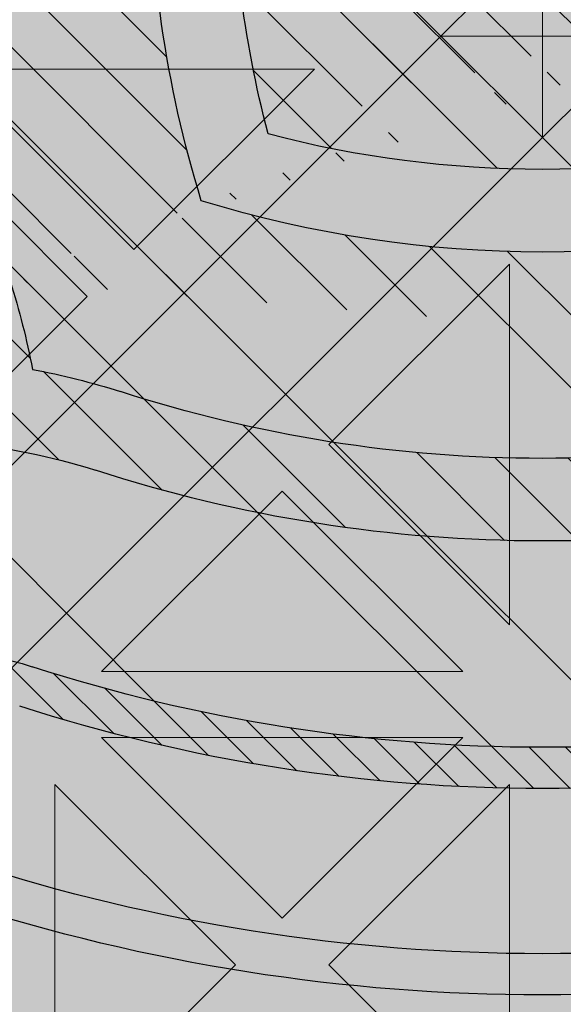
# Model space of a CAD drawing. Units: inches. Extents: x 844 to 2234, y 346 to 1084.
# Tile 28 of 93: x 1255.358 to 1257.455, y 687.38 to 691.183. Entities that reach past the tile are written whole.
import ezdxf

# ---------------------------------------------------------------- set-up
doc = ezdxf.new("R2010")
doc.units = ezdxf.units.IN
doc.header["$MEASUREMENT"] = 0
doc.layers.add('furniture', color=8, linetype='Continuous', lineweight=18)
doc.layers.add('RA-AP-01$0$INT', color=35, linetype='Continuous', lineweight=5)
doc.layers.add('RA-AP-01$0$FURN', color=3, linetype='Continuous')
doc.layers.add('RA-AP-01$0$WOOD', color=64, linetype='Continuous')

# ---------------------------------------------------------------- blocks, each defined once
blk = doc.blocks.new('A$C18D01794')
at = {"layer": 'RA-AP-01$0$INT'}
h = blk.add_hatch(color=256, dxfattribs=at)
h.paths.add_polyline_path([(4.585917135068449, -6.356712009588271), (4.555206456959269, -6.35671200958746), (4.555206456959137, -6.387422687716308), (4.874495778835233, -6.706712009592356), (4.90520645695423, -6.676001331474049)])
h.paths.add_polyline_path([(5.255206456948813, -6.387422687716306), (5.255206456948682, -6.356712009605972), (5.224495778822613, -6.356712009605161), (4.905206456953498, -6.676001331474273), (4.935917135072151, -6.706712009592924)])
h.paths.add_polyline_path([(4.935917135072559, -6.706712009592068), (4.905206456953564, -6.737422687710376), (5.255206456951813, -7.087422687708613), (5.255206456951549, -7.026001331471008)])
h.paths.add_polyline_path([(4.555206456956399, -7.026001331471013), (4.555206456956134, -7.087422687708616), (4.905206456953821, -6.737422687710943), (4.874495778835166, -6.70671200959229)])
h = blk.add_hatch(color=256, dxfattribs=at)
h.paths.add_polyline_path([(4.585917135068448, -6.356712009588273), (4.614201406330596, -6.356712009589021), (4.668846067270487, -6.411356670531338), (4.723490728212344, -6.356712009591912), (4.771774999457151, -6.35671200959319), (4.826419660396886, -6.411356670535356), (4.862780050090322, -6.374996280843536), (4.844495778842715, -6.356712009595112), (4.862780050090411, -6.356712009595595), (4.905206456960182, -6.399138416468211), (4.947632863832445, -6.356712009597838), (4.965917135079675, -6.356712009598322), (4.947632863831759, -6.374996280845421), (4.983993253523576, -6.411356670538857), (5.038637914464627, -6.356712009600247), (5.08692218571208, -6.356712009601523), (5.141566846649976, -6.411356670541852), (5.196211507589851, -6.356712009604411), (5.224495778822615, -6.356712009605161), (4.905206456953975, -6.676001331473793)])
h.paths.add_polyline_path([(4.895206456956031, -6.637717060225675), (4.895206456958921, -6.528427738347902), (4.840561796018589, -6.583072399285802)], flags=16)
h.paths.add_polyline_path([(4.915206456955638, -6.637717060226121), (4.969851117895509, -6.583072399288678), (4.915206456957609, -6.528427738348344)], flags=16)
h.paths.add_polyline_path([(4.826419660395175, -6.568930263661755), (4.881064321335613, -6.514285602723745), (4.771774999456703, -6.514285602720857)], flags=16)
h.paths.add_polyline_path([(4.983993253519558, -6.568930263665262), (5.038637914460456, -6.514285602726792), (4.929348592581548, -6.514285602724816)], flags=16)
h.paths.add_polyline_path([(4.881064321336025, -6.494285602723742), (4.826419660397532, -6.439640941782821), (4.771774999457062, -6.494285602720859)], flags=16)
h.paths.add_polyline_path([(4.929348592582019, -6.494285602724817), (5.038637914460982, -6.494285602726792), (4.983993253522945, -6.439640941786327)], flags=16)
h.paths.add_polyline_path([(4.895206456960191, -6.480143467100443), (4.895206456962115, -6.407422687715913), (4.876922185715016, -6.389138416467584), (4.840561796021581, -6.425498806159401)], flags=16)
h.paths.add_polyline_path([(4.915206456958487, -6.480143467100889), (4.969851117899527, -6.425498806162279), (4.933490728206909, -6.389138416468043), (4.9152064569598, -6.40742268771434)], flags=16)
h.paths.add_polyline_path([(4.757632863832376, -6.480143467096812), (4.812277524772842, -6.425498806158772), (4.757632863834348, -6.370854145217844)], flags=16)
h.paths.add_polyline_path([(4.737632863832376, -6.480143467096286), (4.737632863834348, -6.370854145217375), (4.682988202893906, -6.425498806155385)], flags=16)
h.paths.add_polyline_path([(5.05278005008503, -6.480143467103376), (5.052780050087917, -6.370854145224413), (4.998135389146995, -6.425498806162908)], flags=16)
h.paths.add_polyline_path([(5.072780050085024, -6.480143467103744), (5.127424711025931, -6.42549880616527), (5.072780050087916, -6.370854145224832)], flags=16)
h.paths.add_polyline_path([(4.935917135072783, -6.706712009592292), (5.255206456948811, -6.387422687716309), (5.255206456948932, -6.415706958964177), (5.200561796010279, -6.470351619902839), (5.255206456949403, -6.524996280841948), (5.25520645694961, -6.5732805520894), (5.200561796009787, -6.627925213029239), (5.236922185702417, -6.664285602721864), (5.255206456949919, -6.646001331474357), (5.255206456949998, -6.664285602721898), (5.212780050078687, -6.706712009592262), (5.25520645695036, -6.749138416463932), (5.255206456950438, -6.767422687711313), (5.236922185702424, -6.749138416463297), (5.200561796009796, -6.785498806155928), (5.255206456950753, -6.840143467096874), (5.25520645695096, -6.888427738341682), (5.200561796010322, -6.943072399282328), (5.255206456951428, -6.997717060223427), (5.255206456951547, -7.026001331471006)])
h.paths.add_polyline_path([(5.042988202883395, -6.785498806155427), (5.097632863823085, -6.840143467095101), (5.097632863822622, -6.730854145216193)], flags=16)
h.paths.add_polyline_path([(5.028846067259663, -6.771356670531693), (5.083490728198774, -6.716712009592573), (4.974201406321001, -6.716712009593042)], flags=16)
h.paths.add_polyline_path([(5.117632863823087, -6.840143467095186), (5.172277524762331, -6.785498806155926), (5.11763286382262, -6.730854145216225)], flags=16)
h.paths.add_polyline_path([(5.08349072819877, -6.696712009593886), (5.028846067259652, -6.642067348654775), (4.974201406320998, -6.696712009593438)], flags=16)
h.paths.add_polyline_path([(5.131774999446817, -6.854285602718917), (5.186419660386065, -6.799640941779662), (5.241064321325782, -6.854285602719365)], flags=17)
h.paths.add_polyline_path([(5.131774999446228, -6.716712009592374), (5.186419660386065, -6.771356670532194), (5.222780050079488, -6.734996280838764), (5.204495778832781, -6.716712009592063)], flags=16)
h.paths.add_polyline_path([(5.097632863822613, -6.682569873970264), (5.097632863823061, -6.573280552091354), (5.042988202883383, -6.627925213031044)], flags=16)
h.paths.add_polyline_path([(5.131774999446899, -6.874285602718915), (5.241064321325809, -6.874285602719364), (5.186419660386591, -6.928930263658598)], flags=17)
h.paths.add_polyline_path([(5.131774999446226, -6.696712009594078), (5.204495778830767, -6.696712009594374), (5.22278005007868, -6.67842773834687), (5.186419660386049, -6.642067348654249)], flags=16)
h.paths.add_polyline_path([(5.11763286382262, -6.682569873970225), (5.17227752476232, -6.627925213030515), (5.117632863823064, -6.573280552091267)], flags=16)
h.paths.add_polyline_path([(5.186419660386069, -6.613783077405491), (5.241064321325754, -6.559138416465795), (5.131774999446791, -6.559138416466263)], flags=16)
h.paths.add_polyline_path([(5.131774999446872, -6.539138416466263), (5.24106432132578, -6.539138416465794), (5.186419660386554, -6.484493755526573)], flags=16)
h.paths.add_polyline_path([(5.255206456951811, -7.08742268770861), (5.255206456951895, -7.106712009588038), (4.555206456956052, -7.106712009588038), (4.555206456956136, -7.087422687708617), (4.905206456953973, -6.737422687710788)])
h.paths.add_polyline_path([(4.983993253513404, -6.8444937555241), (4.92934859257295, -6.899138416462108), (5.03863791445186, -6.899138416465014)], flags=16)
h.paths.add_polyline_path([(4.969851117889988, -6.83035161990006), (4.915206456952556, -6.775706958960171), (4.915206456949648, -6.884996280837944)], flags=16)
h.paths.add_polyline_path([(4.929348592572535, -6.919138416462105), (4.983993253511019, -6.973783077403037), (5.038637914451496, -6.919138416465012)], flags=16)
h.paths.add_polyline_path([(5.052780050074912, -6.93328055208906), (4.998135389134438, -6.987925213027088), (5.052780050072919, -7.042569873968025)], flags=16)
h.paths.add_polyline_path([(5.07278005007491, -6.933280552089588), (5.072780050072918, -7.042569873968497), (5.127424711013374, -6.987925213030498)], flags=16)
h.paths.add_polyline_path([(4.89520645695295, -6.775706958959721), (4.840561796013067, -6.830351619897157), (4.895206456950961, -6.884996280837494)], flags=16)
h.paths.add_polyline_path([(4.915206456948365, -6.933280552085403), (4.915206456946434, -7.006001331471951), (4.933490728192729, -7.024285602719066), (4.969851117886972, -6.987925213026453)], flags=16)
h.paths.add_polyline_path([(4.881064321327021, -6.899138416461022), (4.82641966038902, -6.84449375552057), (4.771774999448108, -6.899138416459029)], flags=16)
h.paths.add_polyline_path([(4.895206456950073, -6.933280552084951), (4.840561796009022, -6.987925213023558), (4.876922185700835, -7.024285602716997), (4.895206456948749, -7.006001331469487)], flags=16)
h.paths.add_polyline_path([(4.983993253510392, -7.0020673486505), (4.947632863816944, -7.038427738342319), (4.965917135064043, -7.05671200959023), (5.038637914448995, -7.056712009591555)], flags=16)
h.paths.add_polyline_path([(4.881064321326543, -6.91913841646102), (4.771774999447578, -6.919138416459031), (4.826419660385607, -6.973783077399508)], flags=16)
h.paths.add_polyline_path([(4.905206456946447, -7.014285602717636), (4.862780050074785, -7.056712009588352), (4.947632863816685, -7.056712009589775)], flags=16)
h.paths.add_polyline_path([(5.14156684663679, -7.002067348654549), (5.086922185696452, -7.056712009592438), (5.196211507574223, -7.056712009594425)], flags=16)
h.paths.add_polyline_path([(4.8264196603837, -7.002067348646972), (4.771774999442643, -7.056712009585575), (4.8444957788276, -7.056712009587508), (4.862780050075511, -7.038427738340416)], flags=16)
h.paths.add_polyline_path([(4.812277524760289, -6.98792521302292), (4.757632863822258, -6.933280552082447), (4.757632863819352, -7.042569873961408)], flags=16)
h.paths.add_polyline_path([(4.73763286382226, -6.933280552082079), (4.682988202881349, -6.987925213020536), (4.737632863819352, -7.04256987396099)], flags=16)
h.paths.add_polyline_path([(4.723490728195188, -7.056712009584289), (4.668846067257299, -7.002067348643949), (4.614201406317417, -7.056712009581383)], flags=16)
h.paths.add_polyline_path([(4.597632863829262, -6.706712009592262), (4.555206456957951, -6.664285602721896), (4.555206456958029, -6.646001331474357), (4.573490728205535, -6.664285602721864), (4.609851117898167, -6.627925213029238), (4.555206456958338, -6.573280552089402), (4.555206456958546, -6.524996280841952), (4.60985111789767, -6.470351619902839), (4.555206456959015, -6.415706958964177), (4.555206456959138, -6.387422687716309), (4.874495778835167, -6.70671200959229), (4.5552064569564, -7.026001331471015), (4.555206456956523, -6.997717060223433), (4.609851117897629, -6.94307239928233), (4.555206456956988, -6.888427738341681), (4.555206456957198, -6.840143467096881), (4.609851117898153, -6.78549880615593), (4.573490728205528, -6.749138416463297), (4.555206456957507, -6.76742268771132), (4.555206456957585, -6.749138416463933)])
h.paths.add_polyline_path([(4.712780050085332, -6.730854145216195), (4.712780050084863, -6.840143467095105), (4.767424711024555, -6.785498806155427)], flags=16)
h.paths.add_polyline_path([(4.726922185709173, -6.716712009592573), (4.781566846648288, -6.771356670531693), (4.836211507586949, -6.716712009593043)], flags=16)
h.paths.add_polyline_path([(4.692780050085327, -6.730854145216225), (4.638135389145619, -6.785498806155928), (4.692780050084865, -6.840143467095185)], flags=16)
h.paths.add_polyline_path([(4.726922185709182, -6.696712009593886), (4.836211507586949, -6.696712009593436), (4.7815668466483, -6.642067348654773)], flags=16)
h.paths.add_polyline_path([(4.678637914461726, -6.71671200959237), (4.605917135075169, -6.716712009592063), (4.587632863828464, -6.734996280838766), (4.623993253521887, -6.771356670532195)], flags=16)
h.paths.add_polyline_path([(4.712780050085336, -6.68256987397026), (4.767424711024568, -6.627925213031042), (4.71278005008489, -6.573280552091352)], flags=16)
h.paths.add_polyline_path([(4.678637914461726, -6.696712009594076), (4.623993253521899, -6.642067348654247), (4.587632863829271, -6.67842773834687), (4.605917135077185, -6.696712009594376)], flags=16)
h.paths.add_polyline_path([(4.692780050085336, -6.682569873970228), (4.692780050084889, -6.573280552091267), (4.638135389145632, -6.627925213030515)], flags=16)
h.paths.add_polyline_path([(4.623993253521885, -6.799640941779662), (4.678637914461131, -6.854285602718915), (4.56934859258217, -6.854285602719365)], flags=17)
h.paths.add_polyline_path([(4.623993253521901, -6.613783077405509), (4.678637914461158, -6.559138416466263), (4.569348592582195, -6.559138416465795)], flags=16)
h.paths.add_polyline_path([(4.678637914461051, -6.874285602718915), (4.623993253521361, -6.928930263658598), (4.569348592582143, -6.874285602719364)], flags=17)
h.paths.add_polyline_path([(4.678637914461076, -6.539138416466263), (4.623993253521399, -6.484493755526573), (4.569348592582167, -6.539138416465796)], flags=16)
h = blk.add_hatch(color=256, dxfattribs=at)
h.paths.add_polyline_path([(4.969851117891331, -6.583072399286455), (4.915206456952669, -6.63771706022511), (4.915206456952222, -6.528427738347337)])
h.paths.add_polyline_path([(4.895206456953064, -6.637717060225108), (4.840561796014413, -6.583072399286448), (4.895206456953533, -6.528427738347335)])
h.paths.add_polyline_path([(4.826419660390684, -6.568930263662714), (4.771774999451003, -6.514285602723024), (4.881064321329913, -6.514285602723489)])
h.paths.add_polyline_path([(4.881064321329884, -6.494285602723492), (4.771774999450921, -6.494285602723024), (4.82641966039018, -6.439640941783778)])
h.paths.add_polyline_path([(4.895206456953734, -6.48014346709988), (4.840561796013912, -6.425498806160046), (4.876922185707337, -6.389138416466622), (4.895206456954043, -6.40742268771333)])
h.paths.add_polyline_path([(4.862780050082808, -6.374996280843689), (4.826419660390178, -6.411356670536314), (4.771774999450351, -6.356712009596481), (4.844495778835303, -6.356712009596181)])
h.paths.add_polyline_path([(4.812277524766446, -6.425498806160041), (4.757632863827191, -6.480143467099289), (4.757632863826741, -6.370854145220329)])
h.paths.add_polyline_path([(4.737632863827191, -6.480143467099214), (4.682988202887508, -6.425498806159518), (4.737632863826743, -6.370854145220299)])
h.paths.add_polyline_path([(4.668846067263777, -6.41135667053579), (4.614201406325123, -6.356712009597128), (4.723490728202894, -6.356712009596675)])
h.paths.add_polyline_path([(4.905206456953846, -6.399138416467422), (4.862780050082654, -6.356712009596229), (4.947632863824561, -6.356712009595756)])
h.paths.add_polyline_path([(4.915206456952028, -6.480143467099882), (4.91520645695173, -6.407422687715346), (4.933490728199234, -6.389138416467428), (4.96985111789186, -6.425498806160055)])
h.paths.add_polyline_path([(5.038637914454841, -6.494285602723048), (4.929348592575874, -6.494285602723497), (4.983993253515593, -6.439640941783787)])
h.paths.add_polyline_path([(4.983993253515065, -6.568930263662725), (4.929348592575849, -6.514285602723495), (5.038637914454755, -6.514285602723045)])
h.paths.add_polyline_path([(5.052780050079843, -6.480143467099317), (4.998135389140595, -6.425498806160058), (5.052780050080309, -6.370854145220356)])
h.paths.add_polyline_path([(4.983993253516868, -6.411356670536324), (4.947632863824241, -6.374996280843694), (4.965917135071747, -6.356712009596188), (5.038637914456701, -6.356712009596504)])
h.paths.add_polyline_path([(5.127424711019533, -6.425498806159557), (5.072780050079843, -6.480143467099239), (5.07278005008031, -6.370854145220326)])
h.paths.add_polyline_path([(5.141566846643269, -6.411356670535829), (5.086922185704154, -6.356712009596707), (5.196211507581929, -6.356712009597176)])
h = blk.add_hatch(color=256, dxfattribs=at)
h.paths.add_polyline_path([(5.028846067259997, -6.642067348655121), (4.974201406321342, -6.696712009593783), (5.083490728199115, -6.69671200959423)])
h.paths.add_polyline_path([(4.974201406321344, -6.716712009593388), (5.028846067260004, -6.771356670532039), (5.083490728199117, -6.716712009592919)])
h.paths.add_polyline_path([(5.042988202883738, -6.785498806155768), (5.097632863823428, -6.840143467095449), (5.097632863822963, -6.73085414521654)])
h.paths.add_polyline_path([(5.117632863822961, -6.730854145216568), (5.117632863823428, -6.840143467095531), (5.172277524762674, -6.785498806156272)])
h.paths.add_polyline_path([(5.131774999446572, -6.716712009592718), (5.186419660386406, -6.77135667053254), (5.222780050079831, -6.734996280839116), (5.204495778833122, -6.716712009592409)])
h.paths.add_polyline_path([(5.236922185702764, -6.749138416463644), (5.200561796010139, -6.785498806156274), (5.255206456949971, -6.840143467096101), (5.255206456950271, -6.76742268771115)])
h.paths.add_polyline_path([(5.186419660386412, -6.799640941780006), (5.131774999447164, -6.854285602719262), (5.241064321326123, -6.854285602719711)])
h.paths.add_polyline_path([(5.131774999447238, -6.874285602719261), (5.186419660386934, -6.928930263658944), (5.241064321326153, -6.874285602719709)])
h.paths.add_polyline_path([(5.200561796010663, -6.943072399282675), (5.255206456949324, -6.997717060221329), (5.255206456949777, -6.888427738343558)])
h.paths.add_polyline_path([(5.21278005007903, -6.706712009592607), (5.255206456950223, -6.749138416463798), (5.255206456950696, -6.664285602721891)])
h.paths.add_polyline_path([(5.13177499944657, -6.696712009594424), (5.204495778831106, -6.696712009594723), (5.222780050079024, -6.678427738347219), (5.186419660386397, -6.642067348654592)])
h.paths.add_polyline_path([(5.117632863823405, -6.573280552091611), (5.117632863822955, -6.682569873970578), (5.172277524762665, -6.627925213030859)])
h.paths.add_polyline_path([(5.042988202883727, -6.627925213031387), (5.097632863822957, -6.682569873970603), (5.097632863823407, -6.573280552091697)])
h.paths.add_polyline_path([(5.131774999447135, -6.559138416466609), (5.186419660386394, -6.613783077405857), (5.241064321326097, -6.559138416466144)])
h.paths.add_polyline_path([(5.200561796010128, -6.627925213029584), (5.236922185702758, -6.664285602722211), (5.255206456950264, -6.646001331474705), (5.255206456949948, -6.573280552089752)])
h.paths.add_polyline_path([(5.186419660386895, -6.484493755526919), (5.131774999447213, -6.539138416466609), (5.241064321326127, -6.539138416466142)])
h.paths.add_polyline_path([(5.200561796010624, -6.470351619903183), (5.255206456949745, -6.524996280842298), (5.255206456949276, -6.415706958964523)])
h = blk.add_hatch(color=256, dxfattribs=at)
h.paths.add_polyline_path([(4.905206456953579, -6.70671200959253), (4.905206456953751, -6.676001331474523), (4.874495778835229, -6.706712009592358)])
h.paths.add_polyline_path([(4.935917135071924, -6.706712009592703), (4.905206456953583, -6.706712009592529), (4.90520645695341, -6.737422687710532)])
h = blk.add_hatch(color=256, dxfattribs=at)
h.paths.add_polyline_path([(4.905206456953409, -6.737422687710532), (4.90520645695358, -6.706712009592529), (4.874495778835235, -6.706712009592359)])
h.paths.add_polyline_path([(4.935917135071928, -6.706712009592703), (4.905206456953754, -6.676001331474527), (4.905206456953582, -6.706712009592529)])
for p, q in [((4.905206456953975, -6.676001331473793), (4.585917135071132, -6.356712009590955)), ((4.905206456953975, -6.676001331473793), (5.224495778822613, -6.356712009605161)), ((5.052780050087917, -6.370854145224413), (4.998135389146995, -6.425498806162908)), ((5.052780050085028, -6.480143467103376), (5.052780050087917, -6.370854145224413)), ((4.969851117899529, -6.425498806162279), (4.93349072820771, -6.389138416468842)), ((4.935917135072783, -6.706712009592292), (5.255206456948813, -6.387422687716307)), ((4.9152064569598, -6.407422687715939), (4.915206456958485, -6.480143467100891)), ((4.915206456958485, -6.480143467100891), (4.969851117899529, -6.425498806162277)), ((5.052780050085028, -6.480143467103376), (4.998135389146995, -6.425498806162908)), ((4.92934859258202, -6.494285602724817), (4.983993253522945, -6.439640941786326)), ((5.038637914460983, -6.494285602726792), (4.983993253522945, -6.439640941786326)), ((5.038637914460983, -6.494285602726792), (4.92934859258202, -6.494285602724817)), ((4.929348592581546, -6.514285602724816), (4.983993253519556, -6.568930263665262)), ((5.038637914460456, -6.514285602726792), (4.929348592581546, -6.514285602724816)), ((4.983993253519558, -6.56893026366526), (5.038637914460456, -6.514285602726792)), ((4.915206456957613, -6.52842773834835), (4.969851117895507, -6.583072399288678)), ((4.915206456957609, -6.528427738348348), (4.915206456955636, -6.637717060226119)), ((5.042988202883385, -6.627925213031041), (5.097632863823062, -6.573280552091352)), ((4.915206456955636, -6.637717060226119), (4.969851117895507, -6.583072399288678)), ((5.097632863822615, -6.682569873970262), (5.042988202883383, -6.627925213031042)), ((4.974201406320999, -6.696712009593436), (5.028846067259652, -6.642067348654775)), ((5.083490728198769, -6.696712009593882), (5.028846067259652, -6.642067348654775)), ((4.874495778835233, -6.706712009592356), (4.905206456953753, -6.676001331474525)), ((4.935917135071927, -6.706712009592701), (4.905206456953751, -6.676001331474525)), ((4.905206456953753, -6.676001331474525), (4.905206456953409, -6.737422687710532)), ((5.08349072819877, -6.696712009593886), (4.974201406320999, -6.696712009593436)), ((4.874495778835233, -6.706712009592358), (4.935917135071925, -6.706712009592703)), ((4.935917135071927, -6.706712009592701), (4.905206456953407, -6.737422687710532)), ((4.935917135072783, -6.706712009592292), (5.255206456951548, -7.026001331471007))]:
    blk.add_line(p, q, dxfattribs=at)
blk = doc.blocks.new('A$C32926AE1')
at = {"layer": 'RA-AP-01$0$FURN'}
h = blk.add_hatch(dxfattribs=at)
h.set_pattern_fill('ANSI31', color=256, scale=0.1, style=0)
h.set_pattern_definition([(45, (0, 0), (-0.0088388347648318, 0.0088388347648318), [])])
edge = h.paths.add_edge_path(flags=16)
edge.add_arc((4.904771284329206, 4.246793130718756), 0.2603971832811541, 75.22398030683196, 104.7760196931204)
edge.add_arc((4.904771284329206, 4.246793130718756), 0.2603971832811541, 75.223980306832, 104.77601969312039, ccw=False)
edge = h.paths.add_edge_path(flags=16)
edge.add_arc((4.904771284329206, 4.067062675376612), 0.2603971832811541, 255.2239803068796, 284.776019693168)
edge.add_arc((4.904771284329206, 4.067062675376612), 0.2603971832811541, 255.22398030687958, 284.77601969316805, ccw=False)
edge = h.paths.add_edge_path(flags=0)
edge.add_arc((4.904771284329206, 4.067062675376612), 0.2603971832811541, 255.2239803068796, 284.776019693168)
edge.add_arc((4.904771284329206, 4.067062675376612), 0.2603971832811541, 255.22398030687958, 284.77601969316805, ccw=False)
edge = h.paths.add_edge_path(flags=0)
edge.add_arc((4.904771284329206, 4.067062675376612), 0.2603971832811541, 255.2239803068796, 284.776019693168)
edge.add_arc((4.904771284329206, 4.067062675376612), 0.2603971832811541, 255.22398030687958, 284.77601969316805, ccw=False)
edge = h.paths.add_edge_path()
edge.add_arc((4.604388392048174, 4.588829985554312), 0.1599999999999918, 342.3781640246255, 354.4317409793762)
edge.add_arc((5.090145208887507, 4.43216705527679), 0.3503971832811637, 162.0091218307731, 180.3186872093483)
edge.add_arc((5.205154176610243, 4.588829985554953), 0.1599999999999917, 185.5682590208461, 197.6218359767349)
edge.add_arc((4.904771284329229, 4.246793130718735), 0.3503971832811761, 72.00912183053516, 107.9908781690354)
edge.add_arc((9.535952835716557, 4.28682295566602), 4.798342501046485, 178.2875002453811, 181.5576802719453)
edge.add_arc((4.719397359771122, 4.43216705527679), 0.3503971832811637, 359.6813127906516, 377.9908781692269)
edge.add_arc((9.535967292294904, 4.286822350292874), 4.778371420254705, 178.2965938931842, 181.5667745797229)
edge.add_arc((4.719397359771122, 4.43216705527679), 0.3303971832811637, 359.6813127906516, 377.9908781692269)
edge.add_arc((0.2735752763637294, 4.286822350292874), 4.7783714202547, 358.4332254202771, 361.7034061068158)
edge.add_arc((5.061434214606998, 4.732549947558029), 0.1600000000000254, 252.3781640250584, 264.4317409792362)
edge.add_arc((4.748108354051257, 4.732549947558012), 0.1600000000000541, 275.5682590208426, 287.6218359759532)
edge.add_arc((4.604388392048115, 4.588829985554317), 0.1800000000000505, 342.3567572500182, 349.3735009646207)
edge.add_arc((5.205154176610254, 4.588829985554976), 0.1800000000000069, 190.6264990356027, 197.6432427513933)
edge.add_arc((5.061434214607106, 4.732549947558013), 0.1800000000000424, 252.3567572496606, 259.3735009644582)
edge.add_arc((4.904771284329208, 4.246793130718737), 0.3303971832811676, 71.99844483668534, 108.0015551637021)
edge.add_arc((4.748108354051414, 4.732549947558045), 0.1800000000000547, 280.6264990355479, 287.6432427495938)
edge.add_arc((5.090145208887514, 4.432167055276789), 0.2803971832811691, 162.8706300666893, 180.816523289902)
edge.add_arc((4.719397359771136, 4.432167055276689), 0.2803971832811534, 359.183476710103, 377.1293699333214)
edge.add_arc((4.904771284329222, 4.246793130718737), 0.2803971832811769, 72.87063006672916, 107.1293699332334)
edge.add_arc((5.090145208887522, 4.432167055276788), 0.2603971832811776, 165.2239803068007, 180.9953123810312)
edge.add_arc((4.719397359771141, 4.432167055276699), 0.2603971832811458, 359.0046876189768, 374.7760196932087)
edge.add_arc((5.090145208887507, 4.43216705527679), 0.3303971832811637, 162.0091218307731, 180.3186872093483)
edge.add_arc((9.53595427642584, 4.285015535491528), 4.728345371032053, 178.265043920078, 181.5679956281801)
edge.add_arc((0.2735882922327999, 4.285015535491582), 4.728345371032045, 358.4320043718193, 361.7349560799204)
edge.add_arc((9.535953591267507, 4.284458026472751), 4.708343996644348, 178.2573054306777, 181.5704995759608)
edge.add_arc((0.273588977391114, 4.284458026472785), 4.708343996644358, 358.4295004240388, 361.7426945693213)
edge.add_arc((0.2735889773911131, 4.029397779622582), 4.708343996644359, 358.2573054306787, 361.5704995759613)
edge.add_arc((9.535953591267518, 4.029397779622618), 4.708343996644359, 178.4295004240391, 181.7426945693223)
edge.add_arc((0.2735882922327901, 4.028840270603786), 4.728345371032054, 358.2650439200796, 361.5679956281808)
edge.add_arc((9.53595427642584, 4.028840270603841), 4.728345371032054, 178.4320043718199, 181.7349560799219)
edge.add_arc((0.2735752763637302, 4.027033455802493), 4.778371420254699, 358.2965938931842, 361.5667745797229)
edge.add_arc((4.719397359771122, 3.881688750818578), 0.3303971832811637, 342.0091218307731, 360.3186872093484)
edge.add_arc((5.090145208887507, 3.881688750818578), 0.3303971832811637, 179.6813127906516, 197.9908781692269)
edge.add_arc((9.535967292294904, 4.027033455802493), 4.778371420254705, 178.433225420277, 181.7034061068158)
edge.add_arc((4.719397359771122, 3.881688750818578), 0.3503971832811637, 342.0091218307731, 360.3186872093484)
edge.add_arc((9.53595283571655, 4.027032850429349), 4.79834250104648, 178.4423197280546, 181.7124997546188)
edge.add_arc((4.719397359771141, 3.881688750818669), 0.2603971832811458, 345.2239803067913, 360.9953123810232)
edge.add_arc((5.090145208887522, 3.88168875081858), 0.2603971832811776, 179.0046876189687, 194.7760196931993)
edge.add_arc((4.904771284329222, 4.067062675376631), 0.2803971832811769, 252.8706300667665, 287.1293699332708)
edge.add_arc((4.719397359771136, 3.881688750818678), 0.2803971832811534, 342.8706300666787, 360.8165232898969)
edge.add_arc((5.090145208887514, 3.881688750818579), 0.2803971832811691, 179.183476710098, 197.1293699333106)
edge.add_arc((4.748108354051414, 3.581305858537323), 0.1800000000000547, 72.3567572504062, 79.37350096445199)
edge.add_arc((4.904771284329208, 4.067062675376631), 0.3303971832811676, 251.9984448362979, 288.0015551633146)
edge.add_arc((5.061434214607106, 3.581305858537355), 0.1800000000000424, 100.6264990355418, 107.6432427503394)
edge.add_arc((5.205154176610254, 3.725025820540392), 0.1800000000000069, 162.3567572486066, 169.3735009643972)
edge.add_arc((4.604388392048115, 3.725025820541051), 0.1800000000000505, 10.62649903537925, 17.64324274998182)
edge.add_arc((4.748108354051257, 3.581305858537356), 0.1600000000000541, 72.37816402404681, 84.43174097915735)
edge.add_arc((4.904771284329229, 4.067062675376632), 0.3503971832811761, 252.0091218309645, 287.9908781694648)
edge.add_arc((5.061434214606998, 3.581305858537339), 0.1600000000000254, 95.56825902076373, 107.6218359749416)
edge.add_arc((5.205154176610243, 3.725025820540414), 0.1599999999999917, 162.3781640232651, 174.4317409791539)
edge.add_arc((5.090145208887507, 3.881688750818578), 0.3503971832811637, 179.6813127906516, 197.9908781692269)
edge.add_arc((4.604388392048174, 3.725025820541056), 0.1599999999999918, 5.568259020623824, 17.62183597537444)
edge.add_arc((0.2735897329420762, 4.28682295566602), 4.798342501046482, 358.4423197280547, 361.7124997546188)
edge.add_arc((0.2735897329420691, 4.027032850429348), 4.798342501046489, 358.2875002453812, 361.5576802719453)
at = {"layer": 'RA-AP-01$0$WOOD'}
h = blk.add_hatch(color=256, dxfattribs=at)
h.dxf.hatch_style = 1
h.paths.add_polyline_path([(5.157430609644524, 4.573483066760929, -0.1009492694046607), (5.155401577623758, 4.593365984175333, -0.1842662638101597), (5.172249623284174, 4.638795604568598, 0.2056608120311276), (5.179560981299304, 4.661316324430096, 0.3614336704623542), (5.134352340494423, 4.706524965234944, 0.2056608120311297), (5.111831620632933, 4.699213607219793, -0.1842662638101113), (5.066402000239693, 4.682365561559342, -0.1055311479399994), (5.045656153913092, 4.68467289944697, 0.1567636581983829), (4.763886414745334, 4.684672899446966, -0.1055311479399895), (4.743140568418733, 4.68236556155934, -0.1842662638100833), (4.6977109480255, 4.69921360721979, 0.2056608120302612), (4.675190228164109, 4.706524965234949, 0.3614336704708441), (4.629981587358889, 4.66131632442871, 0.2056608120245944), (4.637292945374126, 4.638795604567974, -0.1842662638101024), (4.654140991034615, 4.59336598417475, -0.1009492694055169), (4.652111959013835, 4.573483066760181, 0.021410119221476), (4.629748025606143, 4.156712009541676, 0.0214101192214795), (4.652111959013809, 3.739940952323101, -0.1009492694059586), (4.654140991034615, 3.720058034908448, -0.1842662638100975), (4.637292945374126, 3.674628414515226, 0.2056608120245705), (4.629981587358889, 3.652107694654492, 0.3614336704708879), (4.675190228164113, 3.606899053848249, 0.2056608120302384), (4.697710948025501, 3.614210411863408, -0.1842662638100995), (4.743140568418738, 3.63105845752386, -0.1055311479402541), (4.763886414745388, 3.628751119636215, 0.1567636581983776), (5.045656153913137, 3.628751119636244, -0.1055311479397538), (5.066402000239692, 3.631058457523857, -0.1842662638101067), (5.111831620632931, 3.614210411863407, 0.2056608120310924), (5.134352340494417, 3.606899053848256, 0.3614336704624001), (5.179560981299307, 3.652107694653103, 0.2056608120311314), (5.172249623284175, 3.6746284145146, -0.1842662638101402), (5.155401577623758, 3.72005803490786, -0.1009492694051366), (5.15743060964455, 3.739940952322354, 0.0214101192215073), (5.179794543052287, 4.156712009541468, 0.0214101192215252)])
h.paths.add_polyline_path([(4.639748609479751, 4.156712009541513, 0.0213537860821624), (4.661970494867118, 3.741887061152232, -0.094075836301374), (4.664143710413708, 3.7196126951003, -0.1824818158568985), (4.644813765429836, 3.668037719127816, 0.2056608120245319), (4.639939526753007, 3.653023905887301, 0.3614336704710246), (4.676106439397173, 3.616856993242342, 0.2056608120302234), (4.691120252638095, 3.621731231919122, -0.1824818158602558), (4.742695228611606, 3.641061176902986, -0.1029891339458722), (4.766991894714349, 3.638256818950944, 0.156709409989566), (5.042550673941472, 3.638256818950105, -0.102989133958497), (5.066847340047078, 3.641061176902949, -0.1824818158594995), (5.118422316020358, 3.621731231919103, 0.2056608120311416), (5.133436129261316, 3.616856993242346, 0.3614336704621468), (5.169603041905217, 3.653023905886178, 0.2056608120310986), (5.164728803228477, 3.668037719127177, -0.1824818158565612), (5.145398858244737, 3.719612695099578, -0.0940758363009313), (5.147572073791232, 3.741887061151398, 0.0213537860822023), (5.169793959178681, 4.156712009541451, 0.0213537860822226), (5.147572073791203, 4.571536957931898, -0.0940758363005034), (5.145398858244737, 4.59381132398362, -0.1824818158565587), (5.164728803228476, 4.645386299956021, 0.2056608120311045), (5.169603041905216, 4.66040011319702, 0.3614336704621845), (5.133436129261313, 4.696567025840856, 0.2056608120310773), (5.118422316020359, 4.691692787164098, -0.182481815859508), (5.066847340047078, 4.67236284218025, -0.1029891339584606), (5.04255067394148, 4.675167200133092, 0.156709409989566), (4.766991894714357, 4.675167200132257, -0.1029891339458842), (4.742695228611611, 4.672362842180213, -0.1824818158602725), (4.691120252638095, 4.691692787164077, 0.2056608120302152), (4.676106439397174, 4.696567025840858, 0.3614336704710363), (4.639939526753005, 4.660400113195899, 0.2056608120245495), (4.644813765429837, 4.645386299955384, -0.1824818158568934), (4.664143710413708, 4.593811323982902, -0.0940758363009187), (4.661970494867149, 4.571536957931074, 0.021353786082177)], flags=16)
h.paths.add_polyline_path([(5.129794543052235, 4.432167055276933, -0.0141661062790638), (5.130152669293814, 4.156927903047693, -0.0141661062790647), (5.129794543052234, 3.881688750818433, -0.0785247771143638), (5.10979738006795, 3.755143611847103, 0.0945969212073497), (5.105408519571111, 3.717898134952927, 0.1043170707844957), (5.116074640131521, 3.670385395016088, 0.1043170707864965), (5.068561900193738, 3.681051515576561, 0.09459692119553), (5.031316423304057, 3.676662655080835, -0.1580239521427272), (4.778226145355827, 3.676662655080367, 0.0945969211986668), (4.740980668464973, 3.681051515576592, 0.1043170707882822), (4.693467928526415, 3.670385395015844, 0.1043170707867916), (4.704134049087309, 3.717898134953662, 0.0945969211972894), (4.69974518859162, 3.755143611844042, -0.0785247771163196), (4.679748025606343, 3.881688750818406, -0.0141661062790663), (4.679389899364763, 4.156927903047693, -0.0141661062790672), (4.679748025606343, 4.432167055276998, -0.0785247771163064), (4.699745188591625, 4.55871219425134, 0.094596921197333), (4.704134049087308, 4.595957671141738, 0.1043170707867205), (4.693467928526416, 4.643470411079523, 0.1043170707882628), (4.740980668464965, 4.632804290518776, 0.0945969211988114), (4.778226145355874, 4.637193151015016, -0.158023952142669), (5.031316423304015, 4.637193151014546, 0.0945969211956361), (5.068561900193736, 4.632804290518806, 0.1043170707864979), (5.11607464013152, 4.643470411079278, 0.1043170707844617), (5.105408519571112, 4.595957671142455, 0.0945969212074597), (5.109797380067959, 4.558712194248236, -0.0785247771143467)], flags=0)
h.paths.add_polyline_path([(5.119794532311105, 4.432259799204851, -0.0142000800617244), (5.120156169157484, 4.156927903047701, -0.0142000800617277), (5.119794532311105, 3.881596006890482, -0.0784894509520253), (5.100273383573699, 3.758192358677797, 0.0940138827242913), (5.095413455884425, 3.717477693979438, 0.0606271852308753), (5.099615656341024, 3.686844378806616, 0.0606271852322524), (5.068982341167493, 3.691046579263239, 0.0940138827010453), (5.028267676478798, 3.686186651576848, -0.1580706864508061), (4.781274892180912, 3.686186651576435, 0.0940138827026903), (4.740560227491556, 3.691046579263279, 0.0606271852339895), (4.709926912317155, 3.686844378806508, 0.0606271852329405), (4.714129112773991, 3.717477693980356, 0.094013882701304), (4.709269185087677, 3.758192358669163, -0.0784894509577193), (4.689748036347473, 3.881596006890469, -0.014200080061729), (4.689386399501094, 4.156927903047709, -0.0142000800617217), (4.689748036347473, 4.432259799204808, -0.078489450957724), (4.709269185087651, 4.555663447426125, 0.0940138827014585), (4.714129112773992, 4.596378112114996, 0.0606271852329731), (4.709926912317154, 4.62701142728886, 0.0606271852340196), (4.74056022749157, 4.622809226832087, 0.0940138827024997), (4.781274892180847, 4.627669154518912, -0.1580706864508359), (5.028267676478777, 4.627669154518526, 0.0940138827010946), (5.068982341167492, 4.622809226832129, 0.060627185232254), (5.099615656341024, 4.627011427288751, 0.0606271852308727), (5.095413455884425, 4.59637811211593, 0.0940138827241088), (5.100273383573675, 4.555663447417647, -0.0784894509520978)], flags=0)
h.paths.add_polyline_path([(5.06978912287499, 4.430218106756144, -0.014241683694547), (5.070173729147532, 4.156927903047672, -0.0142416836945458), (5.06978912287499, 3.883637699339223, -0.0800609523125196), (5.052662118612511, 3.773463122773442, 0.0526421978001116), (5.04590916754064, 3.740550867606997, 0.0526421977992423), (5.012996912374707, 3.73379791653534, -0.1583028414718258), (4.796545656286308, 3.73379791653451, 0.0526421978034211), (4.763633401117837, 3.740550867607021, 0.0526421978018622), (4.756880450045755, 3.773463122774558, -0.0800609523117106), (4.739753445783639, 3.883637699339268, -0.0142416836945435), (4.739368839511098, 4.156927903047671, -0.0142416836945477), (4.739753445783639, 4.430218106756155, -0.0800609523116345), (4.75688045004574, 4.540392683320762, 0.052642197801941), (4.763633401117837, 4.573304938488346, 0.0526421978035071), (4.796545656286361, 4.580057889560873, -0.1583028414717561), (5.012996912374669, 4.580057889560039, 0.0526421977993048), (5.04590916754064, 4.57330493848837, 0.0526421978002057), (5.052662118612529, 4.540392683321868, -0.080060952312477)], flags=0)
h.paths.add_polyline_path([(5.049789715110557, 4.43038092723357, -0.0143097550741839), (5.05018085590259, 4.156927903047715, -0.0143097550741854), (5.049789715110558, 3.883474878861827, -0.0800685599149176), (5.03362098255317, 3.779581877367999, 0.0306258898956367), (5.028241146483733, 3.758218888663947, 0.0306258898977031), (5.006878157778253, 3.75283905259408, -0.1583983521624096), (4.802664410878162, 3.752839052594731, 0.0306258898946014), (4.781301422174808, 3.758218888663924, 0.0306258898967912), (4.775921586105202, 3.779581877368794, -0.080068559914251), (4.759752853548071, 3.883474878861786, -0.0143097550741854), (4.759361712756037, 4.156927903047671, -0.0143097550741854), (4.759752853548071, 4.430380927233557, -0.0800685599142479), (4.775921586105193, 4.534273928726546, 0.0306258898968306), (4.781301422174808, 4.555636917431444, 0.0306258898945754), (4.802664410878143, 4.561016753500631, -0.1583983521624168), (5.006878157778244, 4.561016753501291, 0.0306258898977177), (5.028241146483733, 4.555636917431421, 0.0306258898958182), (5.03362098255321, 4.534273928727244, -0.080068559914796)], flags=0)
h.paths.add_polyline_path([(4.999766070382627, 4.428171244713864, -0.0143443147609634), (5.000198441819402, 4.156927903047689, -0.0143443147609612), (4.999766070382627, 3.885684561381556, -0.0784641635803329), (4.987356730658798, 3.799103304488872, -0.1506053783831347), (4.822185837999821, 3.79910330448882, -0.0784641635803318), (4.809776498276007, 3.885684561381509, -0.014344314760963), (4.809344126839227, 4.156927903047677, -0.0143443147609645), (4.809776498276007, 4.428171244713873, -0.0784641635803192), (4.822185837999822, 4.514752501606549, -0.1506053783831338), (4.987356730658798, 4.514752501606494, -0.078464163580285)], flags=0)
h.paths.add_polyline_path([(4.979755254238824, 4.42764379880488, -0.0143772539198268), (4.980205517789977, 4.156927903047693, -0.0143772539198275), (4.979755254238824, 3.886212007290489, -0.0689242507424422), (4.971183264704897, 3.815276770442801, -0.1296645318904179), (4.838359303953726, 3.815276770442746, -0.0689242507424186), (4.829787314419809, 3.886212007290419, -0.0143772539198292), (4.829337050868653, 4.156927903047653, -0.0143772539198325), (4.829787314419809, 4.427643798804946, -0.0689242507424211), (4.838359303953725, 4.498579035652621, -0.1296645318904187), (4.971183264704897, 4.498579035652565, -0.0689242507424401)], flags=0)
h = blk.add_hatch(color=256, dxfattribs=at)
h.dxf.hatch_style = 1
h.paths.add_polyline_path([(5.145398858244737, 4.59381132398362, -0.1824818158565616), (5.164728803228476, 4.645386299956021, 0.2056608120311045), (5.169603041905216, 4.66040011319702, 0.3614336704621845), (5.133436129261313, 4.696567025840856, 0.2056608120310773), (5.118422316020359, 4.691692787164098, -0.182481815859508), (5.066847340047078, 4.67236284218025, -0.1029891339584606), (5.04255067394148, 4.675167200133092, 0.156709409989566), (4.766991894714357, 4.675167200132257, -0.1029891339458842), (4.742695228611611, 4.672362842180213, -0.1824818158602725), (4.691120252638095, 4.691692787164077, 0.2056608120302152), (4.676106439397174, 4.696567025840858, 0.3614336704710363), (4.639939526753005, 4.660400113195899, 0.2056608120245495), (4.644813765429837, 4.645386299955384, -0.1824818158568934), (4.664143710413708, 4.593811323982902, -0.0940758363009187), (4.661970494867149, 4.571536957931074, 0.0213537860821772), (4.639748609479751, 4.156712009541507, 0.0213537860821625), (4.661970494867119, 3.741887061152226, -0.0940758363013071), (4.664143710413708, 3.719612695100309, -0.1824818158569294), (4.644813765429836, 3.668037719127816, 0.2056608120245319), (4.639939526753007, 3.653023905887301, 0.3614336704710246), (4.676106439397173, 3.616856993242342, 0.2056608120302234), (4.691120252638095, 3.621731231919122, -0.1824818158602558), (4.742695228611606, 3.641061176902986, -0.1029891339458722), (4.766991894714349, 3.638256818950944, 0.156709409989566), (5.042550673941472, 3.638256818950105, -0.102989133958497), (5.066847340047078, 3.641061176902949, -0.1824818158594995), (5.118422316020358, 3.621731231919103, 0.2056608120311416), (5.133436129261316, 3.616856993242346, 0.3614336704621468), (5.169603041905217, 3.653023905886178, 0.2056608120310986), (5.164728803228477, 3.668037719127177, -0.1824818158565612), (5.145398858244737, 3.719612695099578, -0.0940758363009313), (5.147572073791232, 3.741887061151398, 0.0213537860822023), (5.169793959178681, 4.156712009541451, 0.0213537860822226), (5.147572073791203, 4.571536957931898, -0.0940758363004996)])
h.paths.add_polyline_path([(5.109797380067958, 4.55871219424824, -0.0785247771143472), (5.129794543052234, 4.432167055276936, -0.0141661062790644), (5.130152669293814, 4.156927903047685, -0.014166106279066), (5.129794543052234, 3.881688750818401, -0.0785247771143517), (5.109797380067946, 3.755143611847092, 0.0945969212073132), (5.105408519571111, 3.717898134952929, 0.1043170707844995), (5.116074640131521, 3.670385395016088, 0.1043170707864965), (5.068561900193738, 3.681051515576561, 0.09459692119553), (5.031316423304057, 3.676662655080835, -0.1580239521427272), (4.778226145355827, 3.676662655080367, 0.0945969211986668), (4.740980668464973, 3.681051515576592, 0.1043170707882822), (4.693467928526415, 3.670385395015844, 0.1043170707867916), (4.704134049087309, 3.717898134953662, 0.0945969211972894), (4.69974518859162, 3.755143611844042, -0.0785247771163196), (4.679748025606343, 3.881688750818406, -0.0141661062790663), (4.679389899364763, 4.156927903047693, -0.0141661062790672), (4.679748025606343, 4.432167055276998, -0.0785247771163064), (4.699745188591625, 4.55871219425134, 0.094596921197333), (4.704134049087308, 4.595957671141738, 0.1043170707867205), (4.693467928526416, 4.643470411079523, 0.1043170707882628), (4.740980668464965, 4.632804290518776, 0.0945969211988114), (4.778226145355874, 4.637193151015016, -0.158023952142669), (5.031316423304015, 4.637193151014546, 0.0945969211956361), (5.068561900193736, 4.632804290518806, 0.1043170707864979), (5.11607464013152, 4.643470411079278, 0.1043170707844617), (5.105408519571112, 4.595957671142455, 0.0945969212074504)], flags=16)
h.paths.add_polyline_path([(5.100273383573655, 4.55566344741771, -0.0784894509521388), (5.119794532311105, 4.432259799204852, -0.0142000800617252), (5.120156169157484, 4.156927903047686, -0.014200080061726), (5.119794532311105, 3.881596006890502, -0.0784894509520446), (5.100273383573696, 3.758192358677786, 0.0940138827242721), (5.095413455884425, 3.717477693979436, 0.0606271852308692), (5.099615656341024, 3.686844378806616, 0.0606271852322522), (5.068982341167493, 3.691046579263239, 0.0940138827010453), (5.028267676478798, 3.686186651576848, -0.1580706864508061), (4.781274892180912, 3.686186651576435, 0.0940138827026903), (4.740560227491556, 3.691046579263279, 0.0606271852339895), (4.709926912317155, 3.686844378806508, 0.0606271852329405), (4.714129112773991, 3.717477693980356, 0.094013882701304), (4.709269185087677, 3.758192358669163, -0.0784894509577193), (4.689748036347473, 3.881596006890469, -0.014200080061729), (4.689386399501094, 4.156927903047709, -0.0142000800617217), (4.689748036347473, 4.432259799204808, -0.078489450957724), (4.709269185087651, 4.555663447426125, 0.0940138827014585), (4.714129112773992, 4.596378112114996, 0.0606271852329731), (4.709926912317154, 4.62701142728886, 0.0606271852340196), (4.74056022749157, 4.622809226832087, 0.0940138827024997), (4.781274892180847, 4.627669154518912, -0.1580706864508359), (5.028267676478777, 4.627669154518526, 0.0940138827010946), (5.068982341167492, 4.622809226832129, 0.060627185232254), (5.099615656341024, 4.627011427288751, 0.0606271852308727), (5.095413455884425, 4.59637811211593, 0.094013882723957)], flags=0)
h.paths.add_polyline_path([(5.04590916754064, 4.57330493848837, 0.0526421978002057), (5.052662118612529, 4.540392683321868, -0.0800609523124783), (5.06978912287499, 4.430218106756142, -0.0142416836945469), (5.070173729147532, 4.156927903047672, -0.0142416836945458), (5.06978912287499, 3.883637699339223, -0.0800609523125196), (5.052662118612511, 3.773463122773442, 0.0526421978001116), (5.04590916754064, 3.740550867606997, 0.0526421977992423), (5.012996912374707, 3.73379791653534, -0.1583028414718258), (4.796545656286308, 3.73379791653451, 0.0526421978034211), (4.763633401117837, 3.740550867607021, 0.0526421978018622), (4.756880450045755, 3.773463122774558, -0.0800609523117106), (4.739753445783639, 3.883637699339268, -0.0142416836945435), (4.739368839511098, 4.156927903047671, -0.0142416836945477), (4.739753445783639, 4.430218106756155, -0.0800609523116345), (4.75688045004574, 4.540392683320762, 0.052642197801941), (4.763633401117837, 4.573304938488346, 0.0526421978035071), (4.796545656286361, 4.580057889560873, -0.1583028414717561), (5.012996912374669, 4.580057889560039, 0.0526421977993048)], flags=0)
h.paths.add_polyline_path([(5.028241146483733, 4.555636917431422, 0.0306258898956949), (5.033620982553182, 4.534273928727329, -0.0800685599148649), (5.049789715110557, 4.430380927233569, -0.0143097550741839), (5.05018085590259, 4.156927903047715, -0.0143097550741854), (5.049789715110558, 3.883474878861827, -0.0800685599149176), (5.03362098255317, 3.779581877367999, 0.0306258898956367), (5.028241146483733, 3.758218888663947, 0.0306258898977031), (5.006878157778253, 3.75283905259408, -0.1583983521624096), (4.802664410878162, 3.752839052594731, 0.0306258898946014), (4.781301422174808, 3.758218888663924, 0.0306258898967912), (4.775921586105202, 3.779581877368794, -0.080068559914251), (4.759752853548071, 3.883474878861786, -0.0143097550741854), (4.759361712756037, 4.156927903047671, -0.0143097550741854), (4.759752853548071, 4.430380927233557, -0.0800685599142479), (4.775921586105193, 4.534273928726546, 0.0306258898968306), (4.781301422174808, 4.555636917431444, 0.0306258898945754), (4.802664410878143, 4.561016753500631, -0.1583983521624168), (5.006878157778244, 4.561016753501291, 0.0306258898977174)], flags=0)
h.paths.add_polyline_path([(4.987356730658798, 4.514752501606494, -0.0784641635803018), (4.999766070382627, 4.428171244713845, -0.0143443147609637), (5.000198441819402, 4.156927903047665, -0.0143443147609622), (4.999766070382628, 3.885684561381514, -0.0784641635802952), (4.987356730658797, 3.799103304488872, -0.1506053783831338), (4.822185837999821, 3.799103304488819, -0.0784641635803342), (4.809776498276007, 3.885684561381512, -0.0143443147609628), (4.809344126839227, 4.156927903047676, -0.0143443147609646), (4.809776498276007, 4.428171244713873, -0.0784641635803192), (4.822185837999822, 4.514752501606549, -0.1506053783831338)], flags=0)
h.paths.add_polyline_path([(4.971183264704897, 4.498579035652566, -0.0689242507424384), (4.979755254238824, 4.427643798804883, -0.0143772539198276), (4.980205517789977, 4.15692790304768, -0.0143772539198258), (4.979755254238823, 3.88621200729051, -0.0689242507424628), (4.971183264704897, 3.815276770442801, -0.129664531890417), (4.838359303953726, 3.815276770442746, -0.0689242507424186), (4.829787314419809, 3.886212007290419, -0.0143772539198292), (4.829337050868653, 4.156927903047653, -0.0143772539198325), (4.829787314419809, 4.427643798804946, -0.0689242507424211), (4.838359303953725, 4.498579035652621, -0.1296645318904187)], flags=0)
h = blk.add_hatch(dxfattribs=at)
h.set_pattern_fill('ANSI31', color=256, scale=0.05, style=0)
h.set_pattern_definition([(45, (0, 0), (-0.0044194173824159, 0.0044194173824159), [])])
h.paths.add_polyline_path([(5.130152669293814, 4.156927903047704, 0.0141661062790657), (5.129794543052234, 4.432167055276982, 0.0777827904001433), (5.110168979996553, 4.557559993161921, -0.0976515123401879), (5.105408519571111, 4.595957671142454, -0.1043170707844687), (5.116074640131522, 4.64347041107928), (5.099615656341024, 4.627011427288751, 0.0606271852308727), (5.095413455884425, 4.59637811211593, 0.0940138827241088), (5.100273383573675, 4.555663447417647, -0.0784894509520972), (5.119794532311105, 4.432259799204852, -0.0142000800617252), (5.120156169157484, 4.156927903047686, -0.014200080061726), (5.119794532311105, 3.881596006890502, -0.0784894509520446), (5.100273383573696, 3.758192358677786, 0.0940138827242721), (5.095413455884425, 3.717477693979436, 0.0606271852308692), (5.099615656341024, 3.686844378806616), (5.116074640131519, 3.67038539501609, -0.1043170707844594), (5.105408519571112, 3.717898134952912, -0.0976515123401594), (5.11016897999655, 3.756295812933435, 0.0777827904001654), (5.129794543052234, 3.881688750818409, 0.0141661062790665)])
h.paths.add_polyline_path([(5.030164222210597, 3.676291055149937, -0.0976515123472002), (5.068561900193739, 3.681051515576561, -0.1043170707864927), (5.116074640131521, 3.670385395016088), (5.099615656341024, 3.686844378806616, 0.0606271852322522), (5.068982341167493, 3.691046579263239, 0.0940138827010453), (5.028267676478798, 3.686186651576848, -0.1580706864508061), (4.781274892180912, 3.686186651576435, 0.0940138827026903), (4.740560227491556, 3.691046579263279, 0.0606271852339913), (4.709926912317154, 3.686844378806508), (4.693467928526416, 3.670385395015845, -0.1043170707882796), (4.740980668464973, 3.681051515576592, -0.0976515123427246), (4.779378346446416, 3.676291055150394, 0.156512506893803)])
h.paths.add_polyline_path([(4.689748036347473, 3.881596006890472, -0.014200080061729), (4.689386399501094, 4.156927903047712, -0.0142000800617195), (4.689748036347473, 4.432259799204768, -0.078489450957742), (4.709269185087648, 4.555663447426114, 0.0940138827014821), (4.714129112773992, 4.596378112114995, 0.0606271852329748), (4.709926912317154, 4.62701142728886), (4.693467928526414, 4.643470411079524, -0.1043170707867939), (4.704134049087309, 4.595957671141706, -0.09765151234893), (4.699373588660725, 4.557559993157876, 0.0777827903975372), (4.679748025606343, 4.432167055276987, 0.0141661062790675), (4.679389899364763, 4.156927903047675, 0.0141661062790641), (4.679748025606343, 3.88168875081843, 0.0777827903975637), (4.699373588660724, 3.756295812937497, -0.0976515123490278), (4.704134049087308, 3.717898134953629, -0.1043170707867196), (4.693467928526416, 3.670385395015845), (4.709926912317155, 3.686844378806508, 0.0606271852329413), (4.714129112773991, 3.717477693980357, 0.0940138827013084), (4.709269185087676, 3.758192358669166, -0.0784894509577192)])
h.paths.add_polyline_path([(4.779378346446434, 4.63756475094498, -0.0976515123427943), (4.740980668464964, 4.632804290518776, -0.1043170707882609), (4.693467928526416, 4.643470411079523), (4.709926912317154, 4.62701142728886, 0.0606271852340196), (4.74056022749157, 4.622809226832087, 0.0940138827024997), (4.781274892180847, 4.627669154518912, -0.1580706864508359), (5.028267676478777, 4.627669154518526, 0.0940138827010946), (5.068982341167492, 4.622809226832129, 0.060627185232254), (5.099615656341024, 4.627011427288751), (5.116074640131521, 4.643470411079279, -0.1043170707865022), (5.068561900193735, 4.632804290518806, -0.0976515123475899), (5.030164222210446, 4.637564750945479, 0.1565125068936924)])
h = blk.add_hatch(dxfattribs=at)
h.set_pattern_fill('ANSI32', color=256, scale=0.2, style=0)
h.set_pattern_definition([(45, (0, 0), (-0.0530330085889911, 0.0530330085889911), []), (45, (0.035355339, 0), (-0.0530330085889911, 0.0530330085889911), [])])
h.paths.add_polyline_path([(5.119794532311105, 4.432259799204823, 0.0777015974868765), (5.10065834347252, 4.554469821747928, -0.0968902511992216), (5.095413455884425, 4.596378112115931, -0.060627185230871), (5.099615656341024, 4.627011427288751, -0.060627185232254), (5.068982341167492, 4.622809226832129, -0.0968902512198245), (5.027074050790956, 4.628054114423209, 0.1564657949319105), (4.782468517866163, 4.628054114422785, -0.0968902512152247), (4.740560227491555, 4.622809226832088, -0.0606271852339878), (4.709926912317155, 4.627011427288859, -0.0606271852329413), (4.714129112773991, 4.596378112115011, -0.0968902512205338), (4.708884225182929, 4.554469821738175, 0.0777015974804443), (4.689748036347473, 4.43225979920482, 0.0142000800617215), (4.689386399501094, 4.156927903047726, 0.0142000800617273), (4.689748036347473, 3.88159600689052, 0.077701597480541), (4.708884225182985, 3.759385984357019, -0.096890251220082), (4.714129112773992, 3.717477693980371, -0.0606271852329731), (4.709926912317154, 3.686844378806507, -0.060627185233988), (4.740560227491554, 3.691046579263279, -0.0968902512152569), (4.782468517866175, 3.685801691672578, 0.1564657949319236), (5.027074050790988, 3.685801691672169, -0.0968902512197451), (5.068982341167491, 3.691046579263239, -0.0606271852322557), (5.099615656341024, 3.686844378806616, -0.0606271852308727), (5.095413455884425, 3.717477693979438, -0.0968902511991229), (5.100658343472507, 3.7593859843474, 0.0777015974868745), (5.119794532311105, 3.8815960068905, 0.014200080061726), (5.120156169157484, 4.156927903047685, 0.0142000800617238)])
h.paths.add_polyline_path([(5.070173729147531, 4.156927903047684, -0.0142416836945481), (5.06978912287499, 3.883637699339191, -0.0800609523125107), (5.052662118612505, 3.773463122773424, 0.0526421978000811), (5.04590916754064, 3.740550867606997, 0.0526421977993214), (5.012996912374658, 3.733797916535325, -0.1583028414717916), (4.796545656286304, 3.733797916534512, 0.0526421978034138), (4.763633401117837, 3.740550867607021, 0.0526421978018622), (4.756880450045755, 3.773463122774558, -0.0800609523117106), (4.739753445783639, 3.883637699339268, -0.0142416836945435), (4.739368839511098, 4.156927903047671, -0.0142416836945477), (4.739753445783639, 4.430218106756155, -0.0800609523116345), (4.75688045004574, 4.540392683320762, 0.052642197801941), (4.763633401117837, 4.573304938488346, 0.0526421978035071), (4.796545656286361, 4.580057889560873, -0.1583028414717561), (5.012996912374669, 4.580057889560039, 0.0526421977993048), (5.04590916754064, 4.57330493848837, 0.0526421978002057), (5.052662118612529, 4.540392683321868, -0.0800609523124783), (5.06978912287499, 4.430218106756142, -0.0142416836945463)], flags=16)
h.paths.add_polyline_path([(5.050180855902591, 4.156927903047686, -0.0143097550741856), (5.049789715110558, 3.883474878861795, -0.0800685599148126), (5.033620982553202, 3.7795818773681, 0.0306258898957837), (5.028241146483733, 3.758218888663947, 0.0306258898977031), (5.006878157778253, 3.75283905259408, -0.1583983521624096), (4.802664410878162, 3.752839052594731, 0.0306258898946014), (4.781301422174808, 3.758218888663924, 0.0306258898967912), (4.775921586105202, 3.779581877368794, -0.080068559914251), (4.759752853548071, 3.883474878861786, -0.0143097550741854), (4.759361712756037, 4.156927903047671, -0.0143097550741854), (4.759752853548071, 4.430380927233557, -0.0800685599142479), (4.775921586105193, 4.534273928726546, 0.0306258898968306), (4.781301422174808, 4.555636917431444, 0.0306258898945754), (4.802664410878143, 4.561016753500631, -0.1583983521624168), (5.006878157778244, 4.561016753501291, 0.0306258898977177), (5.028241146483733, 4.555636917431421, 0.0306258898958182), (5.03362098255321, 4.534273928727244, -0.0800685599147973), (5.049789715110557, 4.430380927233568, -0.0143097550741854)], flags=0)
h.paths.add_polyline_path([(5.000198441819402, 4.15692790304769, -0.0143443147609622), (4.999766070382627, 3.885684561381539, -0.0784641635803169), (4.987356730658798, 3.799103304488873, -0.1506053783831347), (4.822185837999821, 3.79910330448882, -0.0784641635803318), (4.809776498276007, 3.885684561381509, -0.014344314760963), (4.809344126839227, 4.156927903047677, -0.0143443147609645), (4.809776498276007, 4.428171244713873, -0.0784641635803192), (4.822185837999822, 4.514752501606549, -0.1506053783831338), (4.987356730658798, 4.514752501606494, -0.0784641635803018), (4.999766070382627, 4.428171244713845, -0.0143443147609624)], flags=0)
h.paths.add_polyline_path([(4.980205517789976, 4.156927903047707, -0.0143772539198295), (4.979755254238824, 3.886212007290466, -0.06892425074242), (4.971183264704897, 3.815276770442801, -0.129664531890417), (4.838359303953726, 3.815276770442746, -0.0689242507424186), (4.829787314419809, 3.886212007290419, -0.0143772539198292), (4.829337050868653, 4.156927903047653, -0.0143772539198325), (4.829787314419809, 4.427643798804946, -0.0689242507424211), (4.838359303953725, 4.498579035652621, -0.1296645318904187), (4.971183264704897, 4.498579035652565, -0.0689242507424418), (4.979755254238824, 4.427643798804878, -0.0143772539198259)], flags=0)
for centre, radius, start, end in [((4.719397359771141, 3.881688750818669), 0.2603971832811458, 345.2239803067913, 0.9953123810231653), ((4.719397359771136, 3.881688750818678), 0.2803971832811534, 342.8706300666787, 0.8165232898969792), ((4.904771284329206, 4.067062675376612), 0.2603971832811541, 255.2239803068796, 284.776019693168), ((4.904771284329206, 4.067062675376612), 0.2603971832811541, 255.2239803068796, 284.776019693168), ((4.904771284329222, 4.067062675376631), 0.2803971832811769, 252.8706300667665, 287.1293699332708), ((5.205154176610254, 3.725025820540392), 0.1800000000000069, 162.3567572486066, 169.3735009643972), ((5.061434214607106, 3.581305858537355), 0.1800000000000424, 100.6264990355418, 107.6432427503394), ((4.904771284329208, 4.067062675376631), 0.3303971832811676, 251.9984448362979, 288.0015551633146), ((5.061434214606998, 3.581305858537339), 0.1600000000000254, 95.56825902076373, 107.6218359749416), ((4.904771284329229, 4.067062675376632), 0.3503971832811761, 252.0091218309645, 287.9908781694648), ((5.061434214607086, 3.581305858537378), 0.1100000000000147, 86.06530991086065, 107.5485591618349), ((4.904771284329219, 4.067062675376634), 0.4003971832811741, 252.0350753990311, 287.9649246011635), ((4.904771284329219, 4.067062675376636), 0.4103971832811756, 252.0403002450644, 287.9596997551364), ((4.904771284329217, 4.067062675376635), 0.4503971832811742, 252.0623235132636, 287.9376764870612), ((4.904771284329219, 4.067062675376637), 0.4603971832811766, 252.0683908477148, 287.9316091522846)]:
    blk.add_arc(centre, radius, start, end, dxfattribs=at)
blk = doc.blocks.new('A$C5D2F253E')
at = {"layer": 'RA-AP-01$0$FURN', "xscale": -0.7999999999883585, "yscale": 0.7999999999883585, "zscale": 0.8, "rotation": 90}
blk.add_blockref('A$C18D01794', (-5.687757199772477, 4.75791982714071), dxfattribs=at)
at = {"layer": 'RA-AP-01$0$WOOD', "rotation": 270}
blk.add_blockref('A$C32926AE1', (-4.161339601644158, 5.73852594588169), dxfattribs=at)

msp = doc.modelspace()

# ---------------------------------------------------------------- block references
at = {"layer": 'furniture', "xscale": -15.94108302203742, "yscale": 15.94108302203742, "zscale": 15.94108302203742, "rotation": 270}
msp.add_blockref('A$C5D2F253E', (1244.08405109492, 696.2584716700112), dxfattribs=at)

doc.saveas('drawing.dxf')
